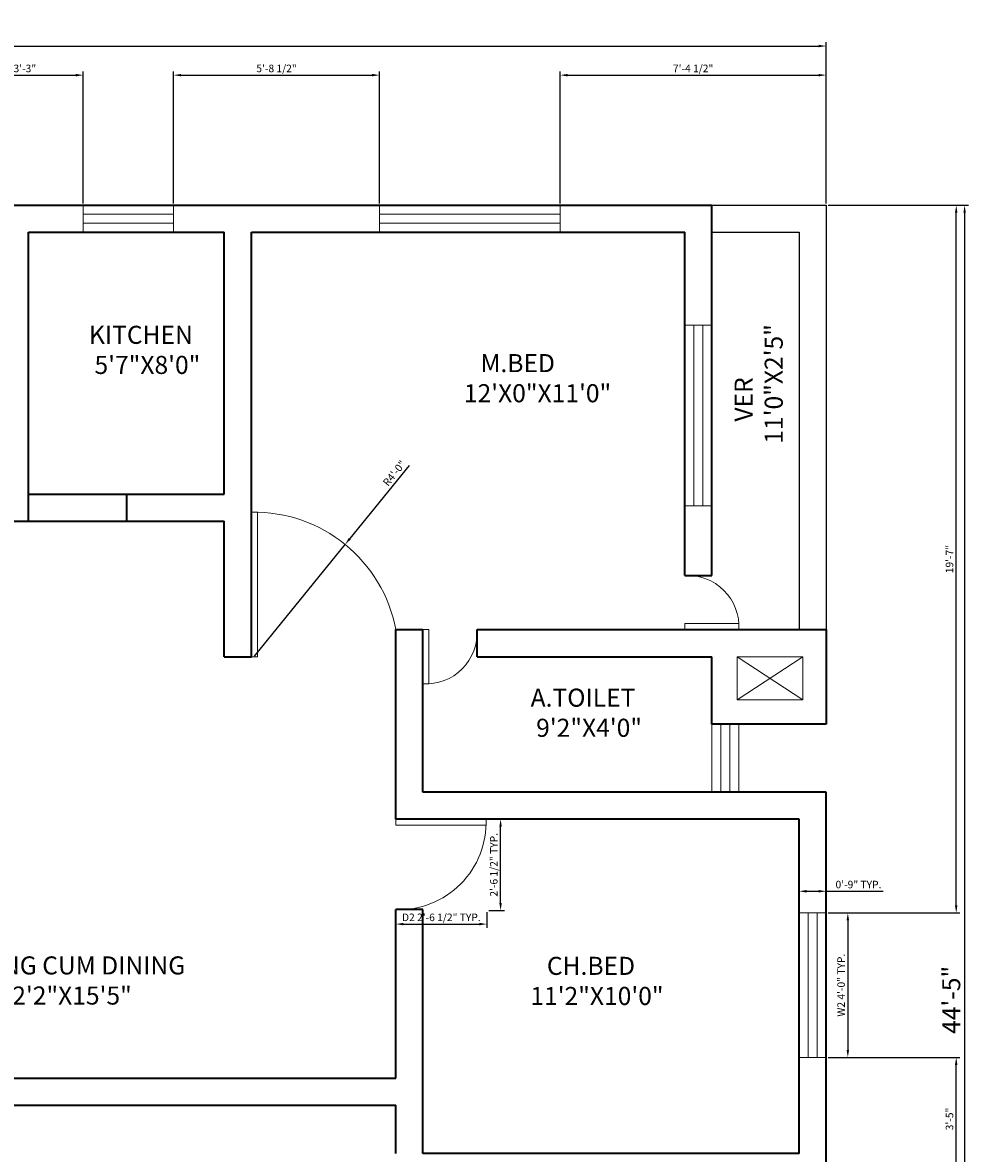
# Model space of a CAD drawing. Units: inches. Extents: x 3941 to 4852, y 2755 to 3388.
# Tile 5 of 5: x 4537 to 4852, y 3013 to 3388. Entities that reach past the tile are written whole.
import ezdxf

# ---------------------------------------------------------------- set-up
doc = ezdxf.new("R2010")
doc.units = ezdxf.units.IN
for name, color, linetype, lineweight in [('A-ANNO-DIMS', 2, 'Continuous', 18), ('A-AREA-IDEN', 7, 'Continuous', 18), ('A-DOOR', 2, 'Continuous', 18), ('A-FLOR-OPEN', 7, 'Continuous', 18), ('A-GLAZ', 5, 'Continuous', 18), ('A-WALL', 7, 'Continuous', 35), ('A-WALL-PRPT', 6, 'Continuous', 25)]:
    doc.layers.add(name, color=color, linetype=linetype, lineweight=lineweight)
doc.styles.get("Standard").update_dxf_attribs({"font": 'arial.ttf'})
doc.dimstyles.new('ISO-25', dxfattribs={"dimtxt": 2.5, "dimasz": 2.5, "dimexe": 1.25, "dimexo": 0.625, "dimtad": 1, "dimlunit": 3, "dimtxsty": 'Standard', "dimcen": 2.5, "dimadec": 0, "dimazin": 0, "dimtfac": 1, "dimtmove": 0, "dimatfit": 3, "dimfxl": 1, "dimarcsym": 0})

# ---------------------------------------------------------------- blocks, each defined once
blk = doc.blocks.new('*D1')
at = {"layer": 'A-ANNO-DIMS', "color": 0, "lineweight": -2, "transparency": 16777216}
for p, q in [((3988.25, 3328.38), (3988.25, 3381.9)), ((4804.25, 3328.38), (4804.25, 3381.9)), ((3990.75, 3380.65), (4801.75, 3380.65))]:
    blk.add_line(p, q, dxfattribs=at)
at = {"layer": 'A-ANNO-DIMS', "color": 0, "transparency": 16777216}
for points in [[(3990.75, 3381.06), (3990.75, 3380.23), (3988.25, 3380.65)], [(4801.75, 3381.06), (4801.75, 3380.23), (4804.25, 3380.65)]]:
    blk.add_solid(points, dxfattribs=at)
at = {"layer": 'Defpoints', "color": 0, "transparency": 16777216}
for p in [(4804.25, 3380.65), (3988.25, 3327.75), (4804.25, 3327.75)]:
    blk.add_point(p, dxfattribs=at)
at = {"layer": 'A-ANNO-DIMS', "color": 0, "transparency": 16777216, "insert": (4396.25, 3384.34), "char_height": 6, "attachment_point": 5}
blk.add_mtext("68'", dxfattribs=at)
blk = doc.blocks.new('*D2')
at = {"layer": 'A-ANNO-DIMS', "color": 0, "lineweight": -2, "transparency": 16777216}
for p, q in [((4804.88, 3327.75), (4851.51, 3327.75)), ((4850.26, 3325.25), (4850.26, 2802.25)), ((4804.88, 2799.75), (4851.51, 2799.75))]:
    blk.add_line(p, q, dxfattribs=at)
at = {"layer": 'A-ANNO-DIMS', "color": 0, "transparency": 16777216}
for points in [[(4849.85, 3325.25), (4850.68, 3325.25), (4850.26, 3327.75)], [(4849.85, 2802.25), (4850.68, 2802.25), (4850.26, 2799.75)]]:
    blk.add_solid(points, dxfattribs=at)
at = {"layer": 'Defpoints', "color": 0, "transparency": 16777216}
for p in [(4804.25, 3327.75), (4804.25, 2799.75), (4850.26, 2799.75)]:
    blk.add_point(p, dxfattribs=at)
at = {"layer": 'A-ANNO-DIMS', "color": 0, "transparency": 16777216, "insert": (4846.59, 3063.75), "char_height": 6, "attachment_point": 5, "rotation": 90}
blk.add_mtext('44\'-5"', dxfattribs=at)
blk = doc.blocks.new('WINDOW-60IN')
for p, q in [((0, 60), (9, 60)), ((0, 60), (0, 0)), ((3, 60), (3, 0)), ((6, 60), (6, 0)), ((9, 0), (9, 60)), ((0, 0), (9, 0))]:
    blk.add_line(p, q)
blk = doc.blocks.new('WINDOW-48IN')
for p, q in [((0, 9), (0, 0)), ((0, 9), (48, 9)), ((48, 9), (48, 0)), ((0, 6), (48, 6)), ((0, 3), (48, 3)), ((48, 0), (0, 0))]:
    blk.add_line(p, q)
blk = doc.blocks.new('WINDOW-30IN')
for p, q in [((0, 0), (0, 9)), ((0, 9), (30, 9)), ((30, 9), (30, 0)), ((0, 6), (30, 6)), ((0, 3), (30, 3)), ((30, 0), (0, 0))]:
    blk.add_line(p, q)
blk = doc.blocks.new('DOOR-SWING-18IN')
for p, q in [((0.03, 0), (0.03, 2)), ((0.03, 2), (18.03, 2)), ((18.03, 0), (0.03, 0)), ((18.03, 2), (18.03, 0))]:
    blk.add_line(p, q)
blk.add_arc((17.03, 1), 17.03, 86.6335, 183.3665)
blk = doc.blocks.new('DOOR-SWING-30IN')
for p, q in [((0, 30.02), (30, 30.02)), ((0, 28.02), (0, 30.02)), ((30, 28.02), (0, 28.02)), ((30, 30.02), (30, 28.02))]:
    blk.add_line(p, q)
blk.add_arc((1, 29.02), 29.02, 268.0251, 1.9749)
blk = doc.blocks.new('*D13')
at = {"layer": 'A-ANNO-DIMS', "color": 0, "lineweight": -2, "transparency": 16777216}
for p, q in [((4661.25, 3092.85), (4661.25, 3087.69)), ((4691.53, 3092.85), (4691.53, 3087.69)), ((4663.75, 3088.94), (4689.03, 3088.94))]:
    blk.add_line(p, q, dxfattribs=at)
at = {"layer": 'A-ANNO-DIMS', "color": 0, "transparency": 16777216}
for points in [[(4663.75, 3089.35), (4663.75, 3088.52), (4661.25, 3088.94)], [(4689.03, 3089.35), (4689.03, 3088.52), (4691.53, 3088.94)]]:
    blk.add_solid(points, dxfattribs=at)
at = {"layer": 'Defpoints', "color": 0, "transparency": 16777216}
for p in [(4661.25, 3093.48), (4691.53, 3093.48), (4691.53, 3088.94)]:
    blk.add_point(p, dxfattribs=at)
at = {"layer": 'A-ANNO-DIMS', "color": 0, "transparency": 16777216, "insert": (4676.39, 3090.85), "char_height": 2.5, "attachment_point": 5}
blk.add_mtext('D2 2\'-6 1/2" TYP.', dxfattribs=at)
blk = doc.blocks.new('*D14')
at = {"layer": 'A-ANNO-DIMS', "color": 0, "lineweight": -2, "transparency": 16777216}
for p, q in [((4692.16, 3123.75), (4697.32, 3123.75)), ((4696.07, 3095.98), (4696.07, 3121.25)), ((4692.16, 3093.48), (4697.32, 3093.48))]:
    blk.add_line(p, q, dxfattribs=at)
at = {"layer": 'A-ANNO-DIMS', "color": 0, "transparency": 16777216}
for points in [[(4695.66, 3121.25), (4696.49, 3121.25), (4696.07, 3123.75)], [(4695.66, 3095.98), (4696.49, 3095.98), (4696.07, 3093.48)]]:
    blk.add_solid(points, dxfattribs=at)
at = {"layer": 'Defpoints', "color": 0, "transparency": 16777216}
for p in [(4691.53, 3123.75), (4696.07, 3123.75), (4691.53, 3093.48)]:
    blk.add_point(p, dxfattribs=at)
at = {"layer": 'A-ANNO-DIMS', "color": 0, "transparency": 16777216, "insert": (4694.15, 3108.62), "char_height": 2.5, "attachment_point": 5, "rotation": 90}
blk.add_mtext('2\'-6 1/2" TYP.', dxfattribs=at)
blk = doc.blocks.new('*D17')
at = {"layer": 'A-ANNO-DIMS', "color": 0, "lineweight": -2, "transparency": 16777216}
for p, q in [((4804.88, 3092.64), (4812.7, 3092.64)), ((4811.45, 3090.14), (4811.45, 3047.14)), ((4804.88, 3044.64), (4812.7, 3044.64))]:
    blk.add_line(p, q, dxfattribs=at)
at = {"layer": 'A-ANNO-DIMS', "color": 0, "transparency": 16777216}
for points in [[(4811.04, 3090.14), (4811.87, 3090.14), (4811.45, 3092.64)], [(4811.04, 3047.14), (4811.87, 3047.14), (4811.45, 3044.64)]]:
    blk.add_solid(points, dxfattribs=at)
at = {"layer": 'Defpoints', "color": 0, "transparency": 16777216}
for p in [(4804.25, 3092.64), (4804.25, 3044.64), (4811.45, 3044.64)]:
    blk.add_point(p, dxfattribs=at)
at = {"layer": 'A-ANNO-DIMS', "color": 0, "transparency": 16777216, "insert": (4809.55, 3068.64), "char_height": 2.5, "attachment_point": 5, "rotation": 90}
blk.add_mtext('W2 4\'-0" TYP.', dxfattribs=at)
blk = doc.blocks.new('*D18')
at = {"layer": 'A-ANNO-DIMS', "color": 0, "lineweight": -2, "transparency": 16777216}
for p, q in [((4795.25, 3093.27), (4795.25, 3101.09)), ((4797.75, 3099.84), (4801.75, 3099.84)), ((4804.25, 3093.27), (4804.25, 3101.09)), ((4804.25, 3099.84), (4823.24, 3099.84))]:
    blk.add_line(p, q, dxfattribs=at)
at = {"layer": 'A-ANNO-DIMS', "color": 0, "transparency": 16777216}
for points in [[(4797.75, 3100.26), (4797.75, 3099.42), (4795.25, 3099.84)], [(4801.75, 3100.26), (4801.75, 3099.42), (4804.25, 3099.84)]]:
    blk.add_solid(points, dxfattribs=at)
at = {"layer": 'Defpoints', "color": 0, "transparency": 16777216}
for p in [(4804.25, 3099.84), (4795.25, 3092.64), (4804.25, 3092.64)]:
    blk.add_point(p, dxfattribs=at)
at = {"layer": 'A-ANNO-DIMS', "color": 0, "transparency": 16777216, "insert": (4815, 3101.74), "char_height": 2.5, "attachment_point": 5}
blk.add_mtext('0\'-9" TYP.', dxfattribs=at)
blk = doc.blocks.new('*D32')
at = {"layer": 'A-ANNO-DIMS', "color": 0, "lineweight": -2, "transparency": 16777216}
for p, q in [((4804.88, 3044.64), (4848.72, 3044.64)), ((4847.47, 3006.25), (4847.47, 3042.14)), ((4804.88, 3003.75), (4848.72, 3003.75))]:
    blk.add_line(p, q, dxfattribs=at)
at = {"layer": 'A-ANNO-DIMS', "color": 0, "transparency": 16777216}
for points in [[(4847.05, 3042.14), (4847.88, 3042.14), (4847.47, 3044.64)], [(4847.05, 3006.25), (4847.88, 3006.25), (4847.47, 3003.75)]]:
    blk.add_solid(points, dxfattribs=at)
at = {"layer": 'Defpoints', "color": 0, "transparency": 16777216}
for p in [(4804.25, 3044.64), (4847.47, 3044.64), (4804.25, 3003.75)]:
    blk.add_point(p, dxfattribs=at)
at = {"layer": 'A-ANNO-DIMS', "color": 0, "transparency": 16777216, "insert": (4845.56, 3024.2), "char_height": 2.5, "attachment_point": 5, "rotation": 90}
blk.add_mtext('3\'-5"', dxfattribs=at)
blk = doc.blocks.new('*D33')
at = {"layer": 'A-ANNO-DIMS', "color": 0, "lineweight": -2, "transparency": 16777216}
for p, q in [((4804.88, 3327.75), (4848.72, 3327.75)), ((4847.47, 3095.14), (4847.47, 3325.25)), ((4804.88, 3092.64), (4848.72, 3092.64))]:
    blk.add_line(p, q, dxfattribs=at)
at = {"layer": 'A-ANNO-DIMS', "color": 0, "transparency": 16777216}
for points in [[(4847.05, 3325.25), (4847.88, 3325.25), (4847.47, 3327.75)], [(4847.05, 3095.14), (4847.88, 3095.14), (4847.47, 3092.64)]]:
    blk.add_solid(points, dxfattribs=at)
at = {"layer": 'Defpoints', "color": 0, "transparency": 16777216}
for p in [(4804.25, 3327.75), (4847.47, 3327.75), (4804.25, 3092.64)]:
    blk.add_point(p, dxfattribs=at)
at = {"layer": 'A-ANNO-DIMS', "color": 0, "transparency": 16777216, "insert": (4845.56, 3210.2), "char_height": 2.5, "attachment_point": 5, "rotation": 90}
blk.add_mtext('19\'-7"', dxfattribs=at)
blk = doc.blocks.new('*D39')
at = {"layer": 'A-ANNO-DIMS', "color": 0, "lineweight": -2, "transparency": 16777216}
for p, q in [((4518.59, 3328.38), (4518.59, 3372.22)), ((4521.09, 3370.97), (4554.9, 3370.97)), ((4557.4, 3328.38), (4557.4, 3372.22))]:
    blk.add_line(p, q, dxfattribs=at)
at = {"layer": 'A-ANNO-DIMS', "color": 0, "transparency": 16777216}
for points in [[(4521.09, 3371.38), (4521.09, 3370.55), (4518.59, 3370.97)], [(4554.9, 3371.38), (4554.9, 3370.55), (4557.4, 3370.97)]]:
    blk.add_solid(points, dxfattribs=at)
at = {"layer": 'Defpoints', "color": 0, "transparency": 16777216}
for p in [(4557.4, 3370.97), (4518.59, 3327.75), (4557.4, 3327.75)]:
    blk.add_point(p, dxfattribs=at)
at = {"layer": 'A-ANNO-DIMS', "color": 0, "transparency": 16777216, "insert": (4538, 3372.87), "char_height": 2.5, "attachment_point": 5}
blk.add_mtext('3\'-3"', dxfattribs=at)
blk = doc.blocks.new('*D40')
at = {"layer": 'A-ANNO-DIMS', "color": 0, "lineweight": -2, "transparency": 16777216}
for p, q in [((4587.4, 3328.38), (4587.4, 3372.22)), ((4589.9, 3370.97), (4653.35, 3370.97)), ((4655.85, 3328.38), (4655.85, 3372.22))]:
    blk.add_line(p, q, dxfattribs=at)
at = {"layer": 'A-ANNO-DIMS', "color": 0, "transparency": 16777216}
for points in [[(4589.9, 3371.38), (4589.9, 3370.55), (4587.4, 3370.97)], [(4653.35, 3371.38), (4653.35, 3370.55), (4655.85, 3370.97)]]:
    blk.add_solid(points, dxfattribs=at)
at = {"layer": 'Defpoints', "color": 0, "transparency": 16777216}
for p in [(4655.85, 3370.97), (4587.4, 3327.75), (4655.85, 3327.75)]:
    blk.add_point(p, dxfattribs=at)
at = {"layer": 'A-ANNO-DIMS', "color": 0, "transparency": 16777216, "insert": (4621.63, 3372.88), "char_height": 2.5, "attachment_point": 5}
blk.add_mtext('5\'-8 1/2"', dxfattribs=at)
blk = doc.blocks.new('*D41')
at = {"layer": 'A-ANNO-DIMS', "color": 0, "lineweight": -2, "transparency": 16777216}
for p, q in [((4715.85, 3328.38), (4715.85, 3372.22)), ((4718.35, 3370.97), (4801.75, 3370.97)), ((4804.25, 3328.38), (4804.25, 3372.22))]:
    blk.add_line(p, q, dxfattribs=at)
at = {"layer": 'A-ANNO-DIMS', "color": 0, "transparency": 16777216}
for points in [[(4718.35, 3371.38), (4718.35, 3370.55), (4715.85, 3370.97)], [(4801.75, 3371.38), (4801.75, 3370.55), (4804.25, 3370.97)]]:
    blk.add_solid(points, dxfattribs=at)
at = {"layer": 'Defpoints', "color": 0, "transparency": 16777216}
for p in [(4804.25, 3370.97), (4715.85, 3327.75), (4804.25, 3327.75)]:
    blk.add_point(p, dxfattribs=at)
at = {"layer": 'A-ANNO-DIMS', "color": 0, "transparency": 16777216, "insert": (4760.05, 3372.88), "char_height": 2.5, "attachment_point": 5}
blk.add_mtext('7\'-4 1/2"', dxfattribs=at)
blk = doc.blocks.new('*D42')
at = {"layer": 'A-ANNO-DIMS', "color": 0, "lineweight": -2, "transparency": 16777216}
for p, q in [((4665.74, 3241.32), (4645.98, 3217)), ((4614.25, 3177.95), (4644.41, 3215.06))]:
    blk.add_line(p, q, dxfattribs=at)
at = {"layer": 'A-ANNO-DIMS', "color": 0, "transparency": 16777216}
blk.add_solid([(4645.66, 3217.26), (4646.31, 3216.74), (4644.41, 3215.06)], dxfattribs=at)
at = {"layer": 'Defpoints', "color": 0, "transparency": 16777216}
for p in [(4644.41, 3215.06), (4614.25, 3177.95)]:
    blk.add_point(p, dxfattribs=at)
at = {"layer": 'A-ANNO-DIMS', "color": 0, "transparency": 16777216, "insert": (4661.02, 3238.53), "char_height": 2.5, "attachment_point": 5, "rotation": 50.9066}
blk.add_mtext('R4\'-0"', dxfattribs=at)

msp = doc.modelspace()

# ---------------------------------------------------------------- linework, layer by layer
at = {"layer": 'A-DOOR'}
for p, q in [((4613.254, 3177.754), (4613.254, 3225.754)), ((4613.254, 3225.754), (4615.254, 3225.754)), ((4615.254, 3225.754), (4615.254, 3177.754)), ((4615.254, 3177.754), (4613.254, 3177.754)), ((4661.254, 3123.754), (4663.254, 3123.754))]:
    msp.add_line(p, q, dxfattribs=at)
msp.add_arc((4614.254, 3177.947), 47.818, 10.61399, 91.19829, dxfattribs=at)
at = {"layer": 'A-FLOR-OPEN'}
for p, q in [((4774.696, 3177.754), (4790.696, 3177.754)), ((4774.696, 3177.754), (4774.696, 3163.435)), ((4774.696, 3163.435), (4796.55, 3177.754)), ((4796.55, 3177.754), (4774.696, 3177.754)), ((4774.696, 3177.754), (4796.55, 3163.435)), ((4790.696, 3177.754), (4796.55, 3177.754)), ((4796.55, 3177.754), (4796.55, 3163.435)), ((4774.696, 3163.435), (4775.59, 3163.435)), ((4796.55, 3163.435), (4775.59, 3163.435))]:
    msp.add_line(p, q, dxfattribs=at)
at = {"layer": 'A-GLAZ'}
for p, q in [((4757.254, 3227.874), (4766.254, 3227.874)), ((4766.254, 3132.754), (4766.254, 3155.383)), ((4766.254, 3155.383), (4775.254, 3155.383)), ((4769.254, 3132.754), (4769.254, 3155.383)), ((4772.254, 3132.754), (4772.254, 3155.383)), ((4775.254, 3155.383), (4775.254, 3132.754)), ((4775.254, 3132.754), (4766.254, 3132.754))]:
    msp.add_line(p, q, dxfattribs=at)
at = {"layer": 'A-WALL'}
for p, q in [((4026.254, 3327.754), (4766.254, 3327.754)), ((4766.254, 3204.754), (4766.254, 3327.754)), ((4539.254, 3222.754), (4539.254, 3318.754)), ((4539.254, 3318.754), (4604.254, 3318.754)), ((4604.254, 3231.754), (4604.254, 3318.754)), ((4613.254, 3177.754), (4613.254, 3318.754)), ((4613.254, 3318.754), (4757.254, 3318.754)), ((4757.254, 3204.754), (4757.254, 3318.754)), ((4539.254, 3231.754), (4604.254, 3231.754)), ((4571.754, 3231.754), (4571.754, 3222.754)), ((4530.254, 3222.754), (4604.254, 3222.754)), ((4604.254, 3177.754), (4604.254, 3222.754)), ((4757.254, 3204.754), (4766.254, 3204.754)), ((4661.254, 3123.754), (4661.254, 3186.754)), ((4661.254, 3186.754), (4670.254, 3186.754)), ((4670.254, 3132.754), (4670.254, 3186.754)), ((4688.254, 3177.754), (4688.254, 3186.754)), ((4688.254, 3186.754), (4804.254, 3186.754)), ((4804.254, 3186.754), (4804.254, 3165.754)), ((4804.254, 3186.754), (4804.254, 3162.754)), ((4604.254, 3177.754), (4613.254, 3177.754)), ((4688.254, 3177.754), (4766.254, 3177.754)), ((4766.254, 3155.383), (4766.254, 3177.754)), ((4804.254, 3162.754), (4804.254, 3155.383)), ((4804.254, 3155.383), (4766.254, 3155.383)), ((4804.254, 3132.754), (4670.254, 3132.754)), ((4804.254, 3003.754), (4804.254, 3132.754)), ((4795.254, 3123.754), (4661.254, 3123.754)), ((4795.254, 3012.754), (4795.254, 3123.754)), ((4670.254, 3093.754), (4661.254, 3093.754)), ((4661.254, 3037.754), (4661.254, 3093.754)), ((4670.254, 3012.754), (4670.254, 3093.754)), ((4482.254, 3037.754), (4661.254, 3037.754)), ((4473.254, 3028.754), (4661.254, 3028.754)), ((4661.254, 3012.754), (4661.254, 3028.754)), ((4795.254, 3012.754), (4670.254, 3012.754))]:
    msp.add_line(p, q, dxfattribs=at)
at = {"layer": 'A-WALL-PRPT'}
for p, q in [((4766.254, 3327.754), (4804.254, 3327.754)), ((4804.254, 3327.754), (4804.254, 3186.754)), ((4766.254, 3318.754), (4795.254, 3318.754)), ((4795.254, 3318.754), (4795.254, 3186.754))]:
    msp.add_line(p, q, dxfattribs=at)

# ---------------------------------------------------------------- block references
at = {"layer": 'A-DOOR', "extrusion": (0, 0, -1), "zscale": -1}
msp.add_blockref('DOOR-SWING-18IN', (-4775.283, 3186.754), dxfattribs=at)
at = {"layer": 'A-DOOR', "extrusion": (0, 0, -1), "zscale": -1, "rotation": 90.00000000000115}
msp.add_blockref('DOOR-SWING-18IN', (-4670.253, 3168.725), dxfattribs=at)
at = {"layer": 'A-DOOR'}
msp.add_blockref('DOOR-SWING-30IN', (4661.254, 3093.738), dxfattribs=at)
at = {"layer": 'A-GLAZ'}
for name, p in [('WINDOW-30IN', (4557.403, 3318.754)), ('WINDOW-60IN', (4757.254, 3227.875))]:
    msp.add_blockref(name, p, dxfattribs=at)
for name, p, rotation in [('WINDOW-60IN', (4655.85, 3327.754), 269.9999999999993), ('WINDOW-48IN', (4795.253, 3092.641), 270.0000000000023)]:
    msp.add_blockref(name, p, dxfattribs=dict(at, rotation=rotation))

# ---------------------------------------------------------------- texts
at = {"layer": 'A-AREA-IDEN', "char_height": 6, "attachment_point": 1}
for s, width, heights, insert in [('    KITCHEN\\P     5\'7"X8\'0"', 69.57529, [0], (4551.975, 3287.7)), ('   M.BED\\P12\'X0"X11\'0"', 69.57529, [0], (4683.88, 3278.3)), ('A.TOILET\\P 9\'2"X4\'0"', 69.57529, [0], (4706.062, 3167.156)), (' LIVING CUM DINING\\P        12\'2"X15\'5"', 233.06976, [115.113], (4514.601, 3078.197)), ('   CH.BED\\P11\'2"X10\'0"', 69.57529, [0], (4705.966, 3078.054))]:
    msp.add_mtext_dynamic_manual_height_columns(s, width=width, gutter_width=12.5, heights=heights, dxfattribs=dict(at, insert=insert))
at = {"layer": 'A-AREA-IDEN', "insert": (4773.831, 3248.533), "char_height": 6, "attachment_point": 1, "rotation": 90}
msp.add_mtext_dynamic_manual_height_columns('    VER\\P11\'0"X2\'5"', width=69.57529, gutter_width=12.5, heights=[0], dxfattribs=at)

# ---------------------------------------------------------------- dimensions: what is measured, and where the dimension line sits
at = {"layer": 'A-ANNO-DIMS'}
for base, p1, p2, override, picture, middle in [((4804.254, 3380.647), (3988.254, 3327.754), (4804.254, 3327.754), {"dimtxt": 6, "dimclrd": 0, "dimclre": 0, "dimclrt": 0}, '*D1', (4396.254, 3384.335)), ((4557.403, 3370.967), (4518.593, 3327.754), (4557.403, 3327.754), {"dimdec": 1, "dimlfac": 1, "dimrnd": 0, "dimzin": 1, "dimdsep": 46, "dimlunit": 4, "dimfrac": 2}, '*D39', (4537.998, 3372.869)), ((4655.85, 3370.967), (4587.403, 3327.754), (4655.85, 3327.754), {"dimdec": 1, "dimlfac": 1, "dimrnd": 0, "dimzin": 1, "dimdsep": 46, "dimlunit": 4, "dimfrac": 2}, '*D40', (4621.626, 3372.884)), ((4804.254, 3370.967), (4715.85, 3327.754), (4804.254, 3327.754), {"dimdec": 1, "dimlfac": 1, "dimrnd": 0, "dimzin": 1, "dimdsep": 46, "dimlunit": 4, "dimfrac": 2}, '*D41', (4760.052, 3372.884))]:
    dim = msp.add_linear_dim(base=base, p1=p1, p2=p2, dimstyle='ISO-25', override=override, dxfattribs=at)
    dim.commit()
    dim.dimension.update_dxf_attribs({"geometry": picture, "text_midpoint": middle})
for base, p1, p2, angle, text, override, picture, middle in [((4850.264, 2799.754), (4804.254, 3327.754), (4804.254, 2799.754), 90, '<>-5"', {"dimtxt": 6, "dimclrd": 0, "dimclre": 0, "dimclrt": 0}, '*D2', (4846.588, 3063.754)), ((4696.072, 3123.754), (4691.531, 3093.477), (4691.531, 3123.754), 90, '<> TYP.', {"dimdec": 1, "dimlfac": 1, "dimrnd": 0, "dimzin": 1, "dimdsep": 46, "dimlunit": 4, "dimfrac": 2}, '*D14', (4694.155, 3108.616)), ((4804.254, 3099.841), (4795.254, 3092.641), (4804.254, 3092.641), 0, '<> TYP.', {"dimdec": 1, "dimlfac": 1, "dimrnd": 0, "dimzin": 1, "dimdsep": 46, "dimlunit": 4, "dimfrac": 2}, '*D18', (4814.998, 3101.743)), ((4811.454, 3044.641), (4804.254, 3092.641), (4804.254, 3044.641), 270, 'W2 <> TYP.', {"dimdec": 1, "dimlfac": 1, "dimrnd": 0, "dimzin": 1, "dimdsep": 46, "dimlunit": 4, "dimfrac": 2}, '*D17', (4809.552, 3068.641))]:
    dim = msp.add_linear_dim(base=base, p1=p1, p2=p2, angle=angle, text=text, dimstyle='ISO-25', override=override, dxfattribs=at)
    dim.commit()
    dim.dimension.update_dxf_attribs({"geometry": picture, "text_midpoint": middle})
for base, p1, p2, picture, middle in [((4847.466, 3327.754), (4804.254, 3092.641), (4804.254, 3327.754), '*D33', (4845.565, 3210.198)), ((4847.466, 3044.641), (4804.254, 3003.754), (4804.254, 3044.641), '*D32', (4845.564, 3024.198))]:
    dim = msp.add_linear_dim(base=base, p1=p1, p2=p2, angle=90, dimstyle='ISO-25', override={"dimdec": 1, "dimlfac": 1, "dimrnd": 0, "dimzin": 1, "dimdsep": 46, "dimlunit": 4, "dimfrac": 2}, dxfattribs=at)
    dim.commit()
    dim.dimension.update_dxf_attribs({"geometry": picture, "text_midpoint": middle})
dim = msp.add_radius_dim(center=(4614.254, 3177.947), mpoint=(4644.407, 3215.059), dimstyle='ISO-25', override={"dimdec": 1, "dimlfac": 1, "dimrnd": 0, "dimzin": 1, "dimdsep": 46, "dimlunit": 4, "dimfrac": 2}, dxfattribs=at)
dim.commit()
dim.dimension.update_dxf_attribs({"geometry": '*D42', "text_midpoint": (4662.499, 3237.327), "dimtype": 164})
dim = msp.add_linear_dim(base=(4691.531, 3088.936), p1=(4661.254, 3093.477), p2=(4691.531, 3093.477), text='D2 <> TYP.', dimstyle='ISO-25', override={"dimdec": 1, "dimlfac": 1, "dimrnd": 0, "dimzin": 1, "dimdsep": 46, "dimlunit": 4, "dimfrac": 2}, dxfattribs=at)
dim.commit()
dim.dimension.update_dxf_attribs({"geometry": '*D13', "text_midpoint": (4676.392, 3090.853)})

doc.saveas('drawing.dxf')
